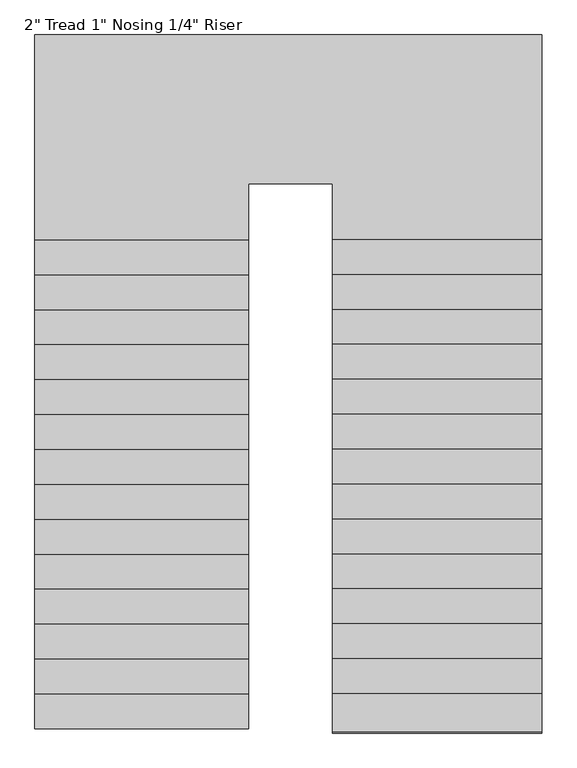
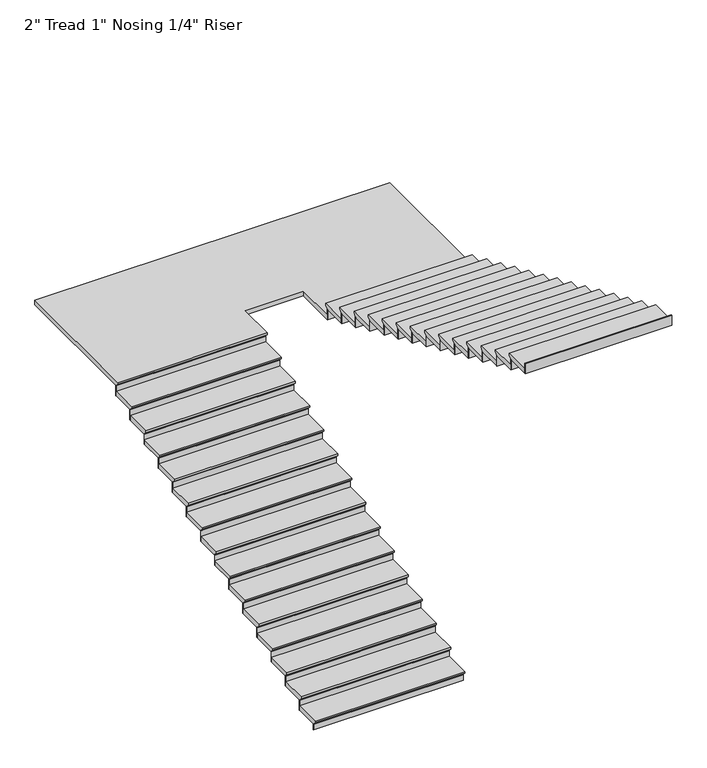
"""IFC4 building model written with IfcOpenShell, lengths in millimetres: stair flight geometry."""

from ifc_helpers import new_model, si_unit, origin, place, context, project, spatial, faceted_brep, source, transform, mapped, element, save


def stair_flight_f7f46773(model_context):
    return source(origin(), model_context, "Body", "Brep", [
        faceted_brep([(-5999.9290366, -6973.0610642, 2835.91), (-5999.9290366, -6973.0610642, 2854.96), (-7554.4415084, -6973.0610642, 2854.96), (-7554.4415084, -6973.0610642, 2835.91), (-5999.9290366, -6947.6610642, 2810.51), (-7554.4415084, -6947.6610642, 2810.51), (-5999.9290366, -6693.6610642, 2854.96), (-7554.4415084, -6693.6610642, 2854.96), (-7554.4415084, -6947.6610642, 2804.16), (-7554.4415084, -6693.6610642, 2804.16), (-5999.9290366, -6693.6610642, 2804.16), (-5999.9290366, -6947.6610642, 2804.16)], [[[0, 1, 2, 3]], [[4, 0, 3, 5]], [[2, 1, 6, 7]], [[8, 9, 10, 11]], [[2, 7, 9, 8, 5, 3]], [[8, 11, 4, 5]], [[6, 1, 0, 4, 11, 10]], [[7, 6, 10, 9]]]),
        faceted_brep([(-5999.9290366, -6947.6610642, 2804.16), (-5999.9290366, -6947.6610642, 2743.2), (-5999.9290366, -6941.3110642, 2743.2), (-5999.9290366, -6941.3110642, 2804.16), (-7554.4415084, -6947.6610642, 2804.16), (-7554.4415084, -6941.3110642, 2804.16), (-7554.4415084, -6941.3110642, 2743.2), (-7554.4415084, -6947.6610642, 2743.2)], [[[0, 1, 2, 3]], [[4, 5, 6, 7]], [[1, 0, 4, 7]], [[2, 1, 7, 6]], [[3, 2, 6, 5]], [[0, 3, 5, 4]]]),
        faceted_brep([(-5999.9290366, -6693.6610642, 2915.92), (-5999.9290366, -6693.6610642, 2804.16), (-5999.9290366, -6687.3110642, 2804.16), (-5999.9290366, -6687.3110642, 2915.92), (-7554.4415084, -6693.6610642, 2915.92), (-7554.4415084, -6687.3110642, 2915.92), (-7554.4415084, -6687.3110642, 2804.16), (-7554.4415084, -6693.6610642, 2804.16)], [[[0, 1, 2, 3]], [[4, 5, 6, 7]], [[1, 0, 4, 7]], [[2, 1, 7, 6]], [[3, 2, 6, 5]], [[0, 3, 5, 4]]]),
        faceted_brep([(-7554.4415084, -6719.0610642, 2966.72), (-5999.9290366, -6719.0610642, 2966.72), (-5999.9290366, -6439.6610642, 2966.72), (-7554.4415084, -6439.6610642, 2966.72), (-7554.4415084, -6693.6610642, 2915.92), (-7554.4415084, -6439.6610642, 2915.92), (-5999.9290366, -6439.6610642, 2915.92), (-5999.9290366, -6693.6610642, 2915.92), (-7554.4415084, -6693.6610642, 2922.27), (-7554.4415084, -6719.0610642, 2947.67), (-5999.9290366, -6693.6610642, 2922.27), (-5999.9290366, -6719.0610642, 2947.67)], [[[0, 1, 2, 3]], [[4, 5, 6, 7]], [[0, 3, 5, 4, 8, 9]], [[4, 7, 10, 8]], [[2, 1, 11, 10, 7, 6]], [[3, 2, 6, 5]], [[11, 1, 0, 9]], [[10, 11, 9, 8]]]),
        faceted_brep([(-5999.9290366, -6439.6610642, 3027.68), (-5999.9290366, -6439.6610642, 2915.92), (-5999.9290366, -6433.3110642, 2915.92), (-5999.9290366, -6433.3110642, 3027.68), (-7554.4415084, -6439.6610642, 3027.68), (-7554.4415084, -6433.3110642, 3027.68), (-7554.4415084, -6433.3110642, 2915.92), (-7554.4415084, -6439.6610642, 2915.92)], [[[0, 1, 2, 3]], [[4, 5, 6, 7]], [[1, 0, 4, 7]], [[2, 1, 7, 6]], [[3, 2, 6, 5]], [[0, 3, 5, 4]]]),
        faceted_brep([(-7554.4415084, -6465.0610642, 3078.48), (-5999.9290366, -6465.0610642, 3078.48), (-5999.9290366, -6185.6610642, 3078.48), (-7554.4415084, -6185.6610642, 3078.48), (-7554.4415084, -6439.6610642, 3027.68), (-7554.4415084, -6185.6610642, 3027.68), (-5999.9290366, -6185.6610642, 3027.68), (-5999.9290366, -6439.6610642, 3027.68), (-7554.4415084, -6439.6610642, 3034.03), (-7554.4415084, -6465.0610642, 3059.43), (-5999.9290366, -6439.6610642, 3034.03), (-5999.9290366, -6465.0610642, 3059.43)], [[[0, 1, 2, 3]], [[4, 5, 6, 7]], [[0, 3, 5, 4, 8, 9]], [[4, 7, 10, 8]], [[2, 1, 11, 10, 7, 6]], [[3, 2, 6, 5]], [[11, 1, 0, 9]], [[10, 11, 9, 8]]]),
        faceted_brep([(-5999.9290366, -6185.6610642, 3139.44), (-5999.9290366, -6185.6610642, 3027.68), (-5999.9290366, -6179.3110642, 3027.68), (-5999.9290366, -6179.3110642, 3139.44), (-7554.4415084, -6185.6610642, 3139.44), (-7554.4415084, -6179.3110642, 3139.44), (-7554.4415084, -6179.3110642, 3027.68), (-7554.4415084, -6185.6610642, 3027.68)], [[[0, 1, 2, 3]], [[4, 5, 6, 7]], [[1, 0, 4, 7]], [[2, 1, 7, 6]], [[3, 2, 6, 5]], [[0, 3, 5, 4]]]),
        faceted_brep([(-7554.4415084, -6211.0610642, 3190.24), (-5999.9290366, -6211.0610642, 3190.24), (-5999.9290366, -5931.6610642, 3190.24), (-7554.4415084, -5931.6610642, 3190.24), (-7554.4415084, -6185.6610642, 3139.44), (-7554.4415084, -5931.6610642, 3139.44), (-5999.9290366, -5931.6610642, 3139.44), (-5999.9290366, -6185.6610642, 3139.44), (-7554.4415084, -6185.6610642, 3145.79), (-7554.4415084, -6211.0610642, 3171.19), (-5999.9290366, -6185.6610642, 3145.79), (-5999.9290366, -6211.0610642, 3171.19)], [[[0, 1, 2, 3]], [[4, 5, 6, 7]], [[0, 3, 5, 4, 8, 9]], [[4, 7, 10, 8]], [[2, 1, 11, 10, 7, 6]], [[3, 2, 6, 5]], [[11, 1, 0, 9]], [[10, 11, 9, 8]]]),
        faceted_brep([(-5999.9290366, -5931.6610642, 3251.2), (-5999.9290366, -5931.6610642, 3139.44), (-5999.9290366, -5925.3110642, 3139.44), (-5999.9290366, -5925.3110642, 3251.2), (-7554.4415084, -5931.6610642, 3251.2), (-7554.4415084, -5925.3110642, 3251.2), (-7554.4415084, -5925.3110642, 3139.44), (-7554.4415084, -5931.6610642, 3139.44)], [[[0, 1, 2, 3]], [[4, 5, 6, 7]], [[1, 0, 4, 7]], [[2, 1, 7, 6]], [[3, 2, 6, 5]], [[0, 3, 5, 4]]]),
        faceted_brep([(-7554.4415084, -5957.0610642, 3302.0), (-5999.9290366, -5957.0610642, 3302.0), (-5999.9290366, -5677.6610642, 3302.0), (-7554.4415084, -5677.6610642, 3302.0), (-7554.4415084, -5931.6610642, 3251.2), (-7554.4415084, -5677.6610642, 3251.2), (-5999.9290366, -5677.6610642, 3251.2), (-5999.9290366, -5931.6610642, 3251.2), (-7554.4415084, -5931.6610642, 3257.55), (-7554.4415084, -5957.0610642, 3282.95), (-5999.9290366, -5931.6610642, 3257.55), (-5999.9290366, -5957.0610642, 3282.95)], [[[0, 1, 2, 3]], [[4, 5, 6, 7]], [[0, 3, 5, 4, 8, 9]], [[4, 7, 10, 8]], [[2, 1, 11, 10, 7, 6]], [[3, 2, 6, 5]], [[11, 1, 0, 9]], [[10, 11, 9, 8]]]),
        faceted_brep([(-5999.9290366, -5677.6610642, 3362.96), (-5999.9290366, -5677.6610642, 3251.2), (-5999.9290366, -5671.3110642, 3251.2), (-5999.9290366, -5671.3110642, 3362.96), (-7554.4415084, -5677.6610642, 3362.96), (-7554.4415084, -5671.3110642, 3362.96), (-7554.4415084, -5671.3110642, 3251.2), (-7554.4415084, -5677.6610642, 3251.2)], [[[0, 1, 2, 3]], [[4, 5, 6, 7]], [[1, 0, 4, 7]], [[2, 1, 7, 6]], [[3, 2, 6, 5]], [[0, 3, 5, 4]]]),
        faceted_brep([(-7554.4415084, -5703.0610642, 3413.76), (-5999.9290366, -5703.0610642, 3413.76), (-5999.9290366, -5423.6610642, 3413.76), (-7554.4415084, -5423.6610642, 3413.76), (-7554.4415084, -5677.6610642, 3362.96), (-7554.4415084, -5423.6610642, 3362.96), (-5999.9290366, -5423.6610642, 3362.96), (-5999.9290366, -5677.6610642, 3362.96), (-7554.4415084, -5677.6610642, 3369.31), (-7554.4415084, -5703.0610642, 3394.71), (-5999.9290366, -5677.6610642, 3369.31), (-5999.9290366, -5703.0610642, 3394.71)], [[[0, 1, 2, 3]], [[4, 5, 6, 7]], [[0, 3, 5, 4, 8, 9]], [[4, 7, 10, 8]], [[2, 1, 11, 10, 7, 6]], [[3, 2, 6, 5]], [[11, 1, 0, 9]], [[10, 11, 9, 8]]]),
        faceted_brep([(-5999.9290366, -5423.6610642, 3474.72), (-5999.9290366, -5423.6610642, 3362.96), (-5999.9290366, -5417.3110642, 3362.96), (-5999.9290366, -5417.3110642, 3474.72), (-7554.4415084, -5423.6610642, 3474.72), (-7554.4415084, -5417.3110642, 3474.72), (-7554.4415084, -5417.3110642, 3362.96), (-7554.4415084, -5423.6610642, 3362.96)], [[[0, 1, 2, 3]], [[4, 5, 6, 7]], [[1, 0, 4, 7]], [[2, 1, 7, 6]], [[3, 2, 6, 5]], [[0, 3, 5, 4]]]),
        faceted_brep([(-7554.4415084, -5449.0610642, 3525.52), (-5999.9290366, -5449.0610642, 3525.52), (-5999.9290366, -5169.6610642, 3525.52), (-7554.4415084, -5169.6610642, 3525.52), (-7554.4415084, -5423.6610642, 3474.72), (-7554.4415084, -5169.6610642, 3474.72), (-5999.9290366, -5169.6610642, 3474.72), (-5999.9290366, -5423.6610642, 3474.72), (-7554.4415084, -5423.6610642, 3481.07), (-7554.4415084, -5449.0610642, 3506.47), (-5999.9290366, -5423.6610642, 3481.07), (-5999.9290366, -5449.0610642, 3506.47)], [[[0, 1, 2, 3]], [[4, 5, 6, 7]], [[0, 3, 5, 4, 8, 9]], [[4, 7, 10, 8]], [[2, 1, 11, 10, 7, 6]], [[3, 2, 6, 5]], [[11, 1, 0, 9]], [[10, 11, 9, 8]]]),
        faceted_brep([(-5999.9290366, -5169.6610642, 3586.48), (-5999.9290366, -5169.6610642, 3474.72), (-5999.9290366, -5163.3110642, 3474.72), (-5999.9290366, -5163.3110642, 3586.48), (-7554.4415084, -5169.6610642, 3586.48), (-7554.4415084, -5163.3110642, 3586.48), (-7554.4415084, -5163.3110642, 3474.72), (-7554.4415084, -5169.6610642, 3474.72)], [[[0, 1, 2, 3]], [[4, 5, 6, 7]], [[1, 0, 4, 7]], [[2, 1, 7, 6]], [[3, 2, 6, 5]], [[0, 3, 5, 4]]]),
        faceted_brep([(-7554.4415084, -5195.0610642, 3637.28), (-5999.9290366, -5195.0610642, 3637.28), (-5999.9290366, -4915.6610642, 3637.28), (-7554.4415084, -4915.6610642, 3637.28), (-7554.4415084, -5169.6610642, 3586.48), (-7554.4415084, -4915.6610642, 3586.48), (-5999.9290366, -4915.6610642, 3586.48), (-5999.9290366, -5169.6610642, 3586.48), (-7554.4415084, -5169.6610642, 3592.83), (-7554.4415084, -5195.0610642, 3618.23), (-5999.9290366, -5169.6610642, 3592.83), (-5999.9290366, -5195.0610642, 3618.23)], [[[0, 1, 2, 3]], [[4, 5, 6, 7]], [[0, 3, 5, 4, 8, 9]], [[4, 7, 10, 8]], [[2, 1, 11, 10, 7, 6]], [[3, 2, 6, 5]], [[11, 1, 0, 9]], [[10, 11, 9, 8]]]),
        faceted_brep([(-5999.9290366, -4915.6610642, 3698.24), (-5999.9290366, -4915.6610642, 3586.48), (-5999.9290366, -4909.3110642, 3586.48), (-5999.9290366, -4909.3110642, 3698.24), (-7554.4415084, -4915.6610642, 3698.24), (-7554.4415084, -4909.3110642, 3698.24), (-7554.4415084, -4909.3110642, 3586.48), (-7554.4415084, -4915.6610642, 3586.48)], [[[0, 1, 2, 3]], [[4, 5, 6, 7]], [[1, 0, 4, 7]], [[2, 1, 7, 6]], [[3, 2, 6, 5]], [[0, 3, 5, 4]]]),
        faceted_brep([(-7554.4415084, -4941.0610642, 3749.04), (-5999.9290366, -4941.0610642, 3749.04), (-5999.9290366, -4661.6610642, 3749.04), (-7554.4415084, -4661.6610642, 3749.04), (-7554.4415084, -4915.6610642, 3698.24), (-7554.4415084, -4661.6610642, 3698.24), (-5999.9290366, -4661.6610642, 3698.24), (-5999.9290366, -4915.6610642, 3698.24), (-7554.4415084, -4915.6610642, 3704.59), (-7554.4415084, -4941.0610642, 3729.99), (-5999.9290366, -4915.6610642, 3704.59), (-5999.9290366, -4941.0610642, 3729.99)], [[[0, 1, 2, 3]], [[4, 5, 6, 7]], [[0, 3, 5, 4, 8, 9]], [[4, 7, 10, 8]], [[2, 1, 11, 10, 7, 6]], [[3, 2, 6, 5]], [[11, 1, 0, 9]], [[10, 11, 9, 8]]]),
        faceted_brep([(-5999.9290366, -4661.6610642, 3810.0), (-5999.9290366, -4661.6610642, 3698.24), (-5999.9290366, -4655.3110642, 3698.24), (-5999.9290366, -4655.3110642, 3810.0), (-7554.4415084, -4661.6610642, 3810.0), (-7554.4415084, -4655.3110642, 3810.0), (-7554.4415084, -4655.3110642, 3698.24), (-7554.4415084, -4661.6610642, 3698.24)], [[[0, 1, 2, 3]], [[4, 5, 6, 7]], [[1, 0, 4, 7]], [[2, 1, 7, 6]], [[3, 2, 6, 5]], [[0, 3, 5, 4]]]),
        faceted_brep([(-7554.4415084, -4687.0610642, 3860.8), (-5999.9290366, -4687.0610642, 3860.8), (-5999.9290366, -4407.6610642, 3860.8), (-7554.4415084, -4407.6610642, 3860.8), (-7554.4415084, -4661.6610642, 3810.0), (-7554.4415084, -4407.6610642, 3810.0), (-5999.9290366, -4407.6610642, 3810.0), (-5999.9290366, -4661.6610642, 3810.0), (-7554.4415084, -4661.6610642, 3816.35), (-7554.4415084, -4687.0610642, 3841.75), (-5999.9290366, -4661.6610642, 3816.35), (-5999.9290366, -4687.0610642, 3841.75)], [[[0, 1, 2, 3]], [[4, 5, 6, 7]], [[0, 3, 5, 4, 8, 9]], [[4, 7, 10, 8]], [[2, 1, 11, 10, 7, 6]], [[3, 2, 6, 5]], [[11, 1, 0, 9]], [[10, 11, 9, 8]]]),
        faceted_brep([(-5999.9290366, -4407.6610642, 3921.76), (-5999.9290366, -4407.6610642, 3810.0), (-5999.9290366, -4401.3110642, 3810.0), (-5999.9290366, -4401.3110642, 3921.76), (-7554.4415084, -4407.6610642, 3921.76), (-7554.4415084, -4401.3110642, 3921.76), (-7554.4415084, -4401.3110642, 3810.0), (-7554.4415084, -4407.6610642, 3810.0)], [[[0, 1, 2, 3]], [[4, 5, 6, 7]], [[1, 0, 4, 7]], [[2, 1, 7, 6]], [[3, 2, 6, 5]], [[0, 3, 5, 4]]]),
        faceted_brep([(-7554.4415084, -4433.0610642, 3972.56), (-5999.9290366, -4433.0610642, 3972.56), (-5999.9290366, -4153.6610642, 3972.56), (-7554.4415084, -4153.6610642, 3972.56), (-7554.4415084, -4407.6610642, 3921.76), (-7554.4415084, -4153.6610642, 3921.76), (-5999.9290366, -4153.6610642, 3921.76), (-5999.9290366, -4407.6610642, 3921.76), (-7554.4415084, -4407.6610642, 3928.11), (-7554.4415084, -4433.0610642, 3953.51), (-5999.9290366, -4407.6610642, 3928.11), (-5999.9290366, -4433.0610642, 3953.51)], [[[0, 1, 2, 3]], [[4, 5, 6, 7]], [[0, 3, 5, 4, 8, 9]], [[4, 7, 10, 8]], [[2, 1, 11, 10, 7, 6]], [[3, 2, 6, 5]], [[11, 1, 0, 9]], [[10, 11, 9, 8]]]),
        faceted_brep([(-5999.9290366, -4153.6610642, 4033.52), (-5999.9290366, -4153.6610642, 3921.76), (-5999.9290366, -4147.3110642, 3921.76), (-5999.9290366, -4147.3110642, 4033.52), (-7554.4415084, -4153.6610642, 4033.52), (-7554.4415084, -4147.3110642, 4033.52), (-7554.4415084, -4147.3110642, 3921.76), (-7554.4415084, -4153.6610642, 3921.76)], [[[0, 1, 2, 3]], [[4, 5, 6, 7]], [[1, 0, 4, 7]], [[2, 1, 7, 6]], [[3, 2, 6, 5]], [[0, 3, 5, 4]]]),
        faceted_brep([(-7554.4415084, -4179.0610642, 4084.32), (-5999.9290366, -4179.0610642, 4084.32), (-5999.9290366, -3899.6610642, 4084.32), (-7554.4415084, -3899.6610642, 4084.32), (-7554.4415084, -4153.6610642, 4033.52), (-7554.4415084, -3899.6610642, 4033.52), (-5999.9290366, -3899.6610642, 4033.52), (-5999.9290366, -4153.6610642, 4033.52), (-7554.4415084, -4153.6610642, 4039.87), (-7554.4415084, -4179.0610642, 4065.27), (-5999.9290366, -4153.6610642, 4039.87), (-5999.9290366, -4179.0610642, 4065.27)], [[[0, 1, 2, 3]], [[4, 5, 6, 7]], [[0, 3, 5, 4, 8, 9]], [[4, 7, 10, 8]], [[2, 1, 11, 10, 7, 6]], [[3, 2, 6, 5]], [[11, 1, 0, 9]], [[10, 11, 9, 8]]]),
        faceted_brep([(-5999.9290366, -3899.6610642, 4145.28), (-5999.9290366, -3899.6610642, 4033.52), (-5999.9290366, -3893.3110642, 4033.52), (-5999.9290366, -3893.3110642, 4145.28), (-7554.4415084, -3899.6610642, 4145.28), (-7554.4415084, -3893.3110642, 4145.28), (-7554.4415084, -3893.3110642, 4033.52), (-7554.4415084, -3899.6610642, 4033.52)], [[[0, 1, 2, 3]], [[4, 5, 6, 7]], [[1, 0, 4, 7]], [[2, 1, 7, 6]], [[3, 2, 6, 5]], [[0, 3, 5, 4]]]),
        faceted_brep([(-7554.4415084, -3925.0610642, 4196.08), (-5999.9290366, -3925.0610642, 4196.08), (-5999.9290366, -3645.6610642, 4196.08), (-7554.4415084, -3645.6610642, 4196.08), (-7554.4415084, -3899.6610642, 4145.28), (-7554.4415084, -3645.6610642, 4145.28), (-5999.9290366, -3645.6610642, 4145.28), (-5999.9290366, -3899.6610642, 4145.28), (-7554.4415084, -3899.6610642, 4151.63), (-7554.4415084, -3925.0610642, 4177.03), (-5999.9290366, -3899.6610642, 4151.63), (-5999.9290366, -3925.0610642, 4177.03)], [[[0, 1, 2, 3]], [[4, 5, 6, 7]], [[0, 3, 5, 4, 8, 9]], [[4, 7, 10, 8]], [[2, 1, 11, 10, 7, 6]], [[3, 2, 6, 5]], [[11, 1, 0, 9]], [[10, 11, 9, 8]]]),
        faceted_brep([(-5999.9290366, -3645.6610642, 4257.04), (-5999.9290366, -3645.6610642, 4145.28), (-5999.9290366, -3639.3110642, 4145.28), (-5999.9290366, -3639.3110642, 4257.04), (-7554.4415084, -3645.6610642, 4257.04), (-7554.4415084, -3639.3110642, 4257.04), (-7554.4415084, -3639.3110642, 4145.28), (-7554.4415084, -3645.6610642, 4145.28)], [[[0, 1, 2, 3]], [[4, 5, 6, 7]], [[1, 0, 4, 7]], [[2, 1, 7, 6]], [[3, 2, 6, 5]], [[0, 3, 5, 4]]]),
        faceted_brep([(-7554.4415084, -3671.0610642, 4307.84), (-5999.9290366, -3671.0610642, 4307.84), (-5999.9290366, -3391.6610642, 4307.84), (-7554.4415084, -3391.6610642, 4307.84), (-7554.4415084, -3645.6610642, 4257.04), (-7554.4415084, -3391.6610642, 4257.04), (-5999.9290366, -3391.6610642, 4257.04), (-5999.9290366, -3645.6610642, 4257.04), (-7554.4415084, -3645.6610642, 4263.39), (-7554.4415084, -3671.0610642, 4288.79), (-5999.9290366, -3645.6610642, 4263.39), (-5999.9290366, -3671.0610642, 4288.79)], [[[0, 1, 2, 3]], [[4, 5, 6, 7]], [[0, 3, 5, 4, 8, 9]], [[4, 7, 10, 8]], [[2, 1, 11, 10, 7, 6]], [[3, 2, 6, 5]], [[11, 1, 0, 9]], [[10, 11, 9, 8]]]),
        faceted_brep([(-5999.9290366, -3391.6610642, 4368.8), (-5999.9290366, -3391.6610642, 4257.04), (-5999.9290366, -3385.3110642, 4257.04), (-5999.9290366, -3385.3110642, 4368.8), (-7554.4415084, -3391.6610642, 4368.8), (-7554.4415084, -3385.3110642, 4368.8), (-7554.4415084, -3385.3110642, 4257.04), (-7554.4415084, -3391.6610642, 4257.04)], [[[0, 1, 2, 3]], [[4, 5, 6, 7]], [[1, 0, 4, 7]], [[2, 1, 7, 6]], [[3, 2, 6, 5]], [[0, 3, 5, 4]]]),
        faceted_brep([(-3866.3290366, -3442.4610642, 4419.6), (-3866.3290366, -1928.4217109, 4419.6), (-7554.4415084, -1928.4217109, 4419.6), (-7554.4415084, -3417.0610642, 4419.6), (-5999.9290366, -3417.0610642, 4419.6), (-5999.9290366, -3010.6610642, 4419.6), (-5390.3290366, -3010.6610642, 4419.6), (-5390.3290366, -3442.4610642, 4419.6), (-3866.3290366, -1928.4217109, 4368.8), (-3866.3290366, -3442.4610642, 4368.8), (-5390.3290366, -3442.4610642, 4368.8), (-5390.3290366, -3010.6610642, 4368.8), (-5999.9290366, -3010.6610642, 4368.8), (-5999.9290366, -3391.6610642, 4368.8), (-7554.4415084, -3391.6610642, 4368.8), (-7554.4415084, -1928.4217109, 4368.8), (-7554.4415084, -3391.6610642, 4375.15), (-7554.4415084, -3417.0610642, 4400.55), (-5999.9290366, -3391.6610642, 4375.15), (-5999.9290366, -3417.0610642, 4400.55)], [[[0, 1, 2, 3, 4, 5, 6, 7]], [[8, 9, 10, 11, 12, 13, 14, 15]], [[1, 0, 9, 8]], [[2, 1, 8, 15]], [[3, 2, 15, 14, 16, 17]], [[14, 13, 18, 16]], [[5, 4, 19, 18, 13, 12]], [[6, 5, 12, 11]], [[7, 6, 11, 10]], [[0, 7, 10, 9]], [[19, 4, 3, 17]], [[18, 19, 17, 16]]]),
        faceted_brep([(-5390.3290366, -3442.4610642, 4480.56), (-5390.3290366, -3442.4610642, 4368.8), (-5390.3290366, -3448.8110642, 4368.8), (-5390.3290366, -3448.8110642, 4480.56), (-3866.3290366, -3442.4610642, 4480.56), (-3866.3290366, -3448.8110642, 4480.56), (-3866.3290366, -3448.8110642, 4368.8), (-3866.3290366, -3442.4610642, 4368.8)], [[[0, 1, 2, 3]], [[4, 5, 6, 7]], [[1, 0, 4, 7]], [[2, 1, 7, 6]], [[3, 2, 6, 5]], [[0, 3, 5, 4]]]),
        faceted_brep([(-3866.3290366, -3417.0610642, 4531.36), (-5390.3290366, -3417.0610642, 4531.36), (-5390.3290366, -3696.4610642, 4531.36), (-3866.3290366, -3696.4610642, 4531.36), (-3866.3290366, -3442.4610642, 4480.56), (-3866.3290366, -3696.4610642, 4480.56), (-5390.3290366, -3696.4610642, 4480.56), (-5390.3290366, -3442.4610642, 4480.56), (-3866.3290366, -3442.4610642, 4486.91), (-3866.3290366, -3417.0610642, 4512.31), (-5390.3290366, -3442.4610642, 4486.91), (-5390.3290366, -3417.0610642, 4512.31)], [[[0, 1, 2, 3]], [[4, 5, 6, 7]], [[0, 3, 5, 4, 8, 9]], [[4, 7, 10, 8]], [[2, 1, 11, 10, 7, 6]], [[3, 2, 6, 5]], [[11, 1, 0, 9]], [[10, 11, 9, 8]]]),
        faceted_brep([(-5390.3290366, -3696.4610642, 4592.32), (-5390.3290366, -3696.4610642, 4480.56), (-5390.3290366, -3702.8110642, 4480.56), (-5390.3290366, -3702.8110642, 4592.32), (-3866.3290366, -3696.4610642, 4592.32), (-3866.3290366, -3702.8110642, 4592.32), (-3866.3290366, -3702.8110642, 4480.56), (-3866.3290366, -3696.4610642, 4480.56)], [[[0, 1, 2, 3]], [[4, 5, 6, 7]], [[1, 0, 4, 7]], [[2, 1, 7, 6]], [[3, 2, 6, 5]], [[0, 3, 5, 4]]]),
        faceted_brep([(-3866.3290366, -3671.0610642, 4643.12), (-5390.3290366, -3671.0610642, 4643.12), (-5390.3290366, -3950.4610642, 4643.12), (-3866.3290366, -3950.4610642, 4643.12), (-3866.3290366, -3696.4610642, 4592.32), (-3866.3290366, -3950.4610642, 4592.32), (-5390.3290366, -3950.4610642, 4592.32), (-5390.3290366, -3696.4610642, 4592.32), (-3866.3290366, -3696.4610642, 4598.67), (-3866.3290366, -3671.0610642, 4624.07), (-5390.3290366, -3696.4610642, 4598.67), (-5390.3290366, -3671.0610642, 4624.07)], [[[0, 1, 2, 3]], [[4, 5, 6, 7]], [[0, 3, 5, 4, 8, 9]], [[4, 7, 10, 8]], [[2, 1, 11, 10, 7, 6]], [[3, 2, 6, 5]], [[11, 1, 0, 9]], [[10, 11, 9, 8]]]),
        faceted_brep([(-5390.3290366, -3950.4610642, 4704.08), (-5390.3290366, -3950.4610642, 4592.32), (-5390.3290366, -3956.8110642, 4592.32), (-5390.3290366, -3956.8110642, 4704.08), (-3866.3290366, -3950.4610642, 4704.08), (-3866.3290366, -3956.8110642, 4704.08), (-3866.3290366, -3956.8110642, 4592.32), (-3866.3290366, -3950.4610642, 4592.32)], [[[0, 1, 2, 3]], [[4, 5, 6, 7]], [[1, 0, 4, 7]], [[2, 1, 7, 6]], [[3, 2, 6, 5]], [[0, 3, 5, 4]]]),
        faceted_brep([(-3866.3290366, -3925.0610642, 4754.88), (-5390.3290366, -3925.0610642, 4754.88), (-5390.3290366, -4204.4610642, 4754.88), (-3866.3290366, -4204.4610642, 4754.88), (-3866.3290366, -3950.4610642, 4704.08), (-3866.3290366, -4204.4610642, 4704.08), (-5390.3290366, -4204.4610642, 4704.08), (-5390.3290366, -3950.4610642, 4704.08), (-3866.3290366, -3950.4610642, 4710.43), (-3866.3290366, -3925.0610642, 4735.83), (-5390.3290366, -3950.4610642, 4710.43), (-5390.3290366, -3925.0610642, 4735.83)], [[[0, 1, 2, 3]], [[4, 5, 6, 7]], [[0, 3, 5, 4, 8, 9]], [[4, 7, 10, 8]], [[2, 1, 11, 10, 7, 6]], [[3, 2, 6, 5]], [[11, 1, 0, 9]], [[10, 11, 9, 8]]]),
        faceted_brep([(-5390.3290366, -4204.4610642, 4815.84), (-5390.3290366, -4204.4610642, 4704.08), (-5390.3290366, -4210.8110642, 4704.08), (-5390.3290366, -4210.8110642, 4815.84), (-3866.3290366, -4204.4610642, 4815.84), (-3866.3290366, -4210.8110642, 4815.84), (-3866.3290366, -4210.8110642, 4704.08), (-3866.3290366, -4204.4610642, 4704.08)], [[[0, 1, 2, 3]], [[4, 5, 6, 7]], [[1, 0, 4, 7]], [[2, 1, 7, 6]], [[3, 2, 6, 5]], [[0, 3, 5, 4]]]),
        faceted_brep([(-3866.3290366, -4179.0610642, 4866.64), (-5390.3290366, -4179.0610642, 4866.64), (-5390.3290366, -4458.4610642, 4866.64), (-3866.3290366, -4458.4610642, 4866.64), (-3866.3290366, -4204.4610642, 4815.84), (-3866.3290366, -4458.4610642, 4815.84), (-5390.3290366, -4458.4610642, 4815.84), (-5390.3290366, -4204.4610642, 4815.84), (-3866.3290366, -4204.4610642, 4822.19), (-3866.3290366, -4179.0610642, 4847.59), (-5390.3290366, -4204.4610642, 4822.19), (-5390.3290366, -4179.0610642, 4847.59)], [[[0, 1, 2, 3]], [[4, 5, 6, 7]], [[0, 3, 5, 4, 8, 9]], [[4, 7, 10, 8]], [[2, 1, 11, 10, 7, 6]], [[3, 2, 6, 5]], [[11, 1, 0, 9]], [[10, 11, 9, 8]]]),
        faceted_brep([(-5390.3290366, -4458.4610642, 4927.6), (-5390.3290366, -4458.4610642, 4815.84), (-5390.3290366, -4464.8110642, 4815.84), (-5390.3290366, -4464.8110642, 4927.6), (-3866.3290366, -4458.4610642, 4927.6), (-3866.3290366, -4464.8110642, 4927.6), (-3866.3290366, -4464.8110642, 4815.84), (-3866.3290366, -4458.4610642, 4815.84)], [[[0, 1, 2, 3]], [[4, 5, 6, 7]], [[1, 0, 4, 7]], [[2, 1, 7, 6]], [[3, 2, 6, 5]], [[0, 3, 5, 4]]]),
        faceted_brep([(-3866.3290366, -4433.0610642, 4978.4), (-5390.3290366, -4433.0610642, 4978.4), (-5390.3290366, -4712.4610642, 4978.4), (-3866.3290366, -4712.4610642, 4978.4), (-3866.3290366, -4458.4610642, 4927.6), (-3866.3290366, -4712.4610642, 4927.6), (-5390.3290366, -4712.4610642, 4927.6), (-5390.3290366, -4458.4610642, 4927.6), (-3866.3290366, -4458.4610642, 4933.95), (-3866.3290366, -4433.0610642, 4959.35), (-5390.3290366, -4458.4610642, 4933.95), (-5390.3290366, -4433.0610642, 4959.35)], [[[0, 1, 2, 3]], [[4, 5, 6, 7]], [[0, 3, 5, 4, 8, 9]], [[4, 7, 10, 8]], [[2, 1, 11, 10, 7, 6]], [[3, 2, 6, 5]], [[11, 1, 0, 9]], [[10, 11, 9, 8]]]),
        faceted_brep([(-5390.3290366, -4712.4610642, 5039.36), (-5390.3290366, -4712.4610642, 4927.6), (-5390.3290366, -4718.8110642, 4927.6), (-5390.3290366, -4718.8110642, 5039.36), (-3866.3290366, -4712.4610642, 5039.36), (-3866.3290366, -4718.8110642, 5039.36), (-3866.3290366, -4718.8110642, 4927.6), (-3866.3290366, -4712.4610642, 4927.6)], [[[0, 1, 2, 3]], [[4, 5, 6, 7]], [[1, 0, 4, 7]], [[2, 1, 7, 6]], [[3, 2, 6, 5]], [[0, 3, 5, 4]]]),
        faceted_brep([(-3866.3290366, -4687.0610642, 5090.16), (-5390.3290366, -4687.0610642, 5090.16), (-5390.3290366, -4966.4610642, 5090.16), (-3866.3290366, -4966.4610642, 5090.16), (-3866.3290366, -4712.4610642, 5039.36), (-3866.3290366, -4966.4610642, 5039.36), (-5390.3290366, -4966.4610642, 5039.36), (-5390.3290366, -4712.4610642, 5039.36), (-3866.3290366, -4712.4610642, 5045.71), (-3866.3290366, -4687.0610642, 5071.11), (-5390.3290366, -4712.4610642, 5045.71), (-5390.3290366, -4687.0610642, 5071.11)], [[[0, 1, 2, 3]], [[4, 5, 6, 7]], [[0, 3, 5, 4, 8, 9]], [[4, 7, 10, 8]], [[2, 1, 11, 10, 7, 6]], [[3, 2, 6, 5]], [[11, 1, 0, 9]], [[10, 11, 9, 8]]]),
        faceted_brep([(-5390.3290366, -4966.4610642, 5151.12), (-5390.3290366, -4966.4610642, 5039.36), (-5390.3290366, -4972.8110642, 5039.36), (-5390.3290366, -4972.8110642, 5151.12), (-3866.3290366, -4966.4610642, 5151.12), (-3866.3290366, -4972.8110642, 5151.12), (-3866.3290366, -4972.8110642, 5039.36), (-3866.3290366, -4966.4610642, 5039.36)], [[[0, 1, 2, 3]], [[4, 5, 6, 7]], [[1, 0, 4, 7]], [[2, 1, 7, 6]], [[3, 2, 6, 5]], [[0, 3, 5, 4]]]),
        faceted_brep([(-3866.3290366, -4941.0610642, 5201.92), (-5390.3290366, -4941.0610642, 5201.92), (-5390.3290366, -5220.4610642, 5201.92), (-3866.3290366, -5220.4610642, 5201.92), (-3866.3290366, -4966.4610642, 5151.12), (-3866.3290366, -5220.4610642, 5151.12), (-5390.3290366, -5220.4610642, 5151.12), (-5390.3290366, -4966.4610642, 5151.12), (-3866.3290366, -4966.4610642, 5157.47), (-3866.3290366, -4941.0610642, 5182.87), (-5390.3290366, -4966.4610642, 5157.47), (-5390.3290366, -4941.0610642, 5182.87)], [[[0, 1, 2, 3]], [[4, 5, 6, 7]], [[0, 3, 5, 4, 8, 9]], [[4, 7, 10, 8]], [[2, 1, 11, 10, 7, 6]], [[3, 2, 6, 5]], [[11, 1, 0, 9]], [[10, 11, 9, 8]]]),
        faceted_brep([(-5390.3290366, -5220.4610642, 5262.88), (-5390.3290366, -5220.4610642, 5151.12), (-5390.3290366, -5226.8110642, 5151.12), (-5390.3290366, -5226.8110642, 5262.88), (-3866.3290366, -5220.4610642, 5262.88), (-3866.3290366, -5226.8110642, 5262.88), (-3866.3290366, -5226.8110642, 5151.12), (-3866.3290366, -5220.4610642, 5151.12)], [[[0, 1, 2, 3]], [[4, 5, 6, 7]], [[1, 0, 4, 7]], [[2, 1, 7, 6]], [[3, 2, 6, 5]], [[0, 3, 5, 4]]]),
        faceted_brep([(-3866.3290366, -5195.0610642, 5313.68), (-5390.3290366, -5195.0610642, 5313.68), (-5390.3290366, -5474.4610642, 5313.68), (-3866.3290366, -5474.4610642, 5313.68), (-3866.3290366, -5220.4610642, 5262.88), (-3866.3290366, -5474.4610642, 5262.88), (-5390.3290366, -5474.4610642, 5262.88), (-5390.3290366, -5220.4610642, 5262.88), (-3866.3290366, -5220.4610642, 5269.23), (-3866.3290366, -5195.0610642, 5294.63), (-5390.3290366, -5220.4610642, 5269.23), (-5390.3290366, -5195.0610642, 5294.63)], [[[0, 1, 2, 3]], [[4, 5, 6, 7]], [[0, 3, 5, 4, 8, 9]], [[4, 7, 10, 8]], [[2, 1, 11, 10, 7, 6]], [[3, 2, 6, 5]], [[11, 1, 0, 9]], [[10, 11, 9, 8]]]),
        faceted_brep([(-5390.3290366, -5474.4610642, 5374.64), (-5390.3290366, -5474.4610642, 5262.88), (-5390.3290366, -5480.8110642, 5262.88), (-5390.3290366, -5480.8110642, 5374.64), (-3866.3290366, -5474.4610642, 5374.64), (-3866.3290366, -5480.8110642, 5374.64), (-3866.3290366, -5480.8110642, 5262.88), (-3866.3290366, -5474.4610642, 5262.88)], [[[0, 1, 2, 3]], [[4, 5, 6, 7]], [[1, 0, 4, 7]], [[2, 1, 7, 6]], [[3, 2, 6, 5]], [[0, 3, 5, 4]]]),
        faceted_brep([(-3866.3290366, -5449.0610642, 5425.44), (-5390.3290366, -5449.0610642, 5425.44), (-5390.3290366, -5728.4610642, 5425.44), (-3866.3290366, -5728.4610642, 5425.44), (-3866.3290366, -5474.4610642, 5374.64), (-3866.3290366, -5728.4610642, 5374.64), (-5390.3290366, -5728.4610642, 5374.64), (-5390.3290366, -5474.4610642, 5374.64), (-3866.3290366, -5474.4610642, 5380.99), (-3866.3290366, -5449.0610642, 5406.39), (-5390.3290366, -5474.4610642, 5380.99), (-5390.3290366, -5449.0610642, 5406.39)], [[[0, 1, 2, 3]], [[4, 5, 6, 7]], [[0, 3, 5, 4, 8, 9]], [[4, 7, 10, 8]], [[2, 1, 11, 10, 7, 6]], [[3, 2, 6, 5]], [[11, 1, 0, 9]], [[10, 11, 9, 8]]]),
        faceted_brep([(-5390.3290366, -5728.4610642, 5486.4), (-5390.3290366, -5728.4610642, 5374.64), (-5390.3290366, -5734.8110642, 5374.64), (-5390.3290366, -5734.8110642, 5486.4), (-3866.3290366, -5728.4610642, 5486.4), (-3866.3290366, -5734.8110642, 5486.4), (-3866.3290366, -5734.8110642, 5374.64), (-3866.3290366, -5728.4610642, 5374.64)], [[[0, 1, 2, 3]], [[4, 5, 6, 7]], [[1, 0, 4, 7]], [[2, 1, 7, 6]], [[3, 2, 6, 5]], [[0, 3, 5, 4]]]),
        faceted_brep([(-3866.3290366, -5703.0610642, 5537.2), (-5390.3290366, -5703.0610642, 5537.2), (-5390.3290366, -5982.4610642, 5537.2), (-3866.3290366, -5982.4610642, 5537.2), (-3866.3290366, -5728.4610642, 5486.4), (-3866.3290366, -5982.4610642, 5486.4), (-5390.3290366, -5982.4610642, 5486.4), (-5390.3290366, -5728.4610642, 5486.4), (-3866.3290366, -5728.4610642, 5492.75), (-3866.3290366, -5703.0610642, 5518.15), (-5390.3290366, -5728.4610642, 5492.75), (-5390.3290366, -5703.0610642, 5518.15)], [[[0, 1, 2, 3]], [[4, 5, 6, 7]], [[0, 3, 5, 4, 8, 9]], [[4, 7, 10, 8]], [[2, 1, 11, 10, 7, 6]], [[3, 2, 6, 5]], [[11, 1, 0, 9]], [[10, 11, 9, 8]]]),
        faceted_brep([(-5390.3290366, -5982.4610642, 5598.16), (-5390.3290366, -5982.4610642, 5486.4), (-5390.3290366, -5988.8110642, 5486.4), (-5390.3290366, -5988.8110642, 5598.16), (-3866.3290366, -5982.4610642, 5598.16), (-3866.3290366, -5988.8110642, 5598.16), (-3866.3290366, -5988.8110642, 5486.4), (-3866.3290366, -5982.4610642, 5486.4)], [[[0, 1, 2, 3]], [[4, 5, 6, 7]], [[1, 0, 4, 7]], [[2, 1, 7, 6]], [[3, 2, 6, 5]], [[0, 3, 5, 4]]]),
        faceted_brep([(-3866.3290366, -5957.0610642, 5648.96), (-5390.3290366, -5957.0610642, 5648.96), (-5390.3290366, -6236.4610642, 5648.96), (-3866.3290366, -6236.4610642, 5648.96), (-3866.3290366, -5982.4610642, 5598.16), (-3866.3290366, -6236.4610642, 5598.16), (-5390.3290366, -6236.4610642, 5598.16), (-5390.3290366, -5982.4610642, 5598.16), (-3866.3290366, -5982.4610642, 5604.51), (-3866.3290366, -5957.0610642, 5629.91), (-5390.3290366, -5982.4610642, 5604.51), (-5390.3290366, -5957.0610642, 5629.91)], [[[0, 1, 2, 3]], [[4, 5, 6, 7]], [[0, 3, 5, 4, 8, 9]], [[4, 7, 10, 8]], [[2, 1, 11, 10, 7, 6]], [[3, 2, 6, 5]], [[11, 1, 0, 9]], [[10, 11, 9, 8]]]),
        faceted_brep([(-5390.3290366, -6236.4610642, 5709.92), (-5390.3290366, -6236.4610642, 5598.16), (-5390.3290366, -6242.8110642, 5598.16), (-5390.3290366, -6242.8110642, 5709.92), (-3866.3290366, -6236.4610642, 5709.92), (-3866.3290366, -6242.8110642, 5709.92), (-3866.3290366, -6242.8110642, 5598.16), (-3866.3290366, -6236.4610642, 5598.16)], [[[0, 1, 2, 3]], [[4, 5, 6, 7]], [[1, 0, 4, 7]], [[2, 1, 7, 6]], [[3, 2, 6, 5]], [[0, 3, 5, 4]]]),
        faceted_brep([(-3866.3290366, -6211.0610642, 5760.72), (-5390.3290366, -6211.0610642, 5760.72), (-5390.3290366, -6490.4610642, 5760.72), (-3866.3290366, -6490.4610642, 5760.72), (-3866.3290366, -6236.4610642, 5709.92), (-3866.3290366, -6490.4610642, 5709.92), (-5390.3290366, -6490.4610642, 5709.92), (-5390.3290366, -6236.4610642, 5709.92), (-3866.3290366, -6236.4610642, 5716.27), (-3866.3290366, -6211.0610642, 5741.67), (-5390.3290366, -6236.4610642, 5716.27), (-5390.3290366, -6211.0610642, 5741.67)], [[[0, 1, 2, 3]], [[4, 5, 6, 7]], [[0, 3, 5, 4, 8, 9]], [[4, 7, 10, 8]], [[2, 1, 11, 10, 7, 6]], [[3, 2, 6, 5]], [[11, 1, 0, 9]], [[10, 11, 9, 8]]]),
        faceted_brep([(-5390.3290366, -6490.4610642, 5821.68), (-5390.3290366, -6490.4610642, 5709.92), (-5390.3290366, -6496.8110642, 5709.92), (-5390.3290366, -6496.8110642, 5821.68), (-3866.3290366, -6490.4610642, 5821.68), (-3866.3290366, -6496.8110642, 5821.68), (-3866.3290366, -6496.8110642, 5709.92), (-3866.3290366, -6490.4610642, 5709.92)], [[[0, 1, 2, 3]], [[4, 5, 6, 7]], [[1, 0, 4, 7]], [[2, 1, 7, 6]], [[3, 2, 6, 5]], [[0, 3, 5, 4]]]),
        faceted_brep([(-3866.3290366, -6465.0610642, 5872.48), (-5390.3290366, -6465.0610642, 5872.48), (-5390.3290366, -6744.4610642, 5872.48), (-3866.3290366, -6744.4610642, 5872.48), (-3866.3290366, -6490.4610642, 5821.68), (-3866.3290366, -6744.4610642, 5821.68), (-5390.3290366, -6744.4610642, 5821.68), (-5390.3290366, -6490.4610642, 5821.68), (-3866.3290366, -6490.4610642, 5828.03), (-3866.3290366, -6465.0610642, 5853.43), (-5390.3290366, -6490.4610642, 5828.03), (-5390.3290366, -6465.0610642, 5853.43)], [[[0, 1, 2, 3]], [[4, 5, 6, 7]], [[0, 3, 5, 4, 8, 9]], [[4, 7, 10, 8]], [[2, 1, 11, 10, 7, 6]], [[3, 2, 6, 5]], [[11, 1, 0, 9]], [[10, 11, 9, 8]]]),
        faceted_brep([(-5390.3290366, -6744.4610642, 5933.44), (-5390.3290366, -6744.4610642, 5821.68), (-5390.3290366, -6750.8110642, 5821.68), (-5390.3290366, -6750.8110642, 5933.44), (-3866.3290366, -6744.4610642, 5933.44), (-3866.3290366, -6750.8110642, 5933.44), (-3866.3290366, -6750.8110642, 5821.68), (-3866.3290366, -6744.4610642, 5821.68)], [[[0, 1, 2, 3]], [[4, 5, 6, 7]], [[1, 0, 4, 7]], [[2, 1, 7, 6]], [[3, 2, 6, 5]], [[0, 3, 5, 4]]]),
        faceted_brep([(-5390.3290366, -6998.4610642, 6045.2), (-5390.3290366, -6998.4610642, 5933.44), (-5390.3290366, -7004.8110642, 5933.44), (-5390.3290366, -7004.8110642, 6045.2), (-3866.3290366, -6998.4610642, 6045.2), (-3866.3290366, -7004.8110642, 6045.2), (-3866.3290366, -7004.8110642, 5933.44), (-3866.3290366, -6998.4610642, 5933.44)], [[[0, 1, 2, 3]], [[4, 5, 6, 7]], [[1, 0, 4, 7]], [[2, 1, 7, 6]], [[3, 2, 6, 5]], [[0, 3, 5, 4]]]),
        faceted_brep([(-3866.3290366, -6719.0610642, 5984.24), (-5390.3290366, -6719.0610642, 5984.24), (-5390.3290366, -6998.4610642, 5984.24), (-3866.3290366, -6998.4610642, 5984.24), (-3866.3290366, -6744.4610642, 5933.44), (-3866.3290366, -6998.4610642, 5933.44), (-5390.3290366, -6998.4610642, 5933.44), (-5390.3290366, -6744.4610642, 5933.44), (-3866.3290366, -6744.4610642, 5939.79), (-3866.3290366, -6719.0610642, 5965.19), (-5390.3290366, -6744.4610642, 5939.79), (-5390.3290366, -6719.0610642, 5965.19)], [[[0, 1, 2, 3]], [[4, 5, 6, 7]], [[0, 3, 5, 4, 8, 9]], [[4, 7, 10, 8]], [[2, 1, 11, 10, 7, 6]], [[3, 2, 6, 5]], [[11, 1, 0, 9]], [[10, 11, 9, 8]]]),
    ])


if __name__ == "__main__":
    model = new_model("IFC4")
    model_context = context("Model", 3, world=origin())
    ifc_project = project(units=[si_unit("LENGTHUNIT", "METRE", prefix="MILLI")], contexts=[model_context])
    site = spatial("IfcSite", under=ifc_project)
    building = spatial("IfcBuilding", under=site)
    placement = place(None, origin())
    stair_flight_shape = stair_flight_f7f46773(model_context)
    element("IfcStairFlight", 1, ObjectType="2\" Tread 1\" Nosing 1/4\" Riser", at=placement, inside=building, context=model_context, shape_type="MappedRepresentation", body=[
        mapped(stair_flight_shape, transform((0.0, 0.0, 0.0), x_axis=(1.0, 0.0, 0.0), y_axis=(0.0, 1.0, 0.0), z_axis=(0.0, 0.0, 1.0))),
    ])
    save(model, "model.ifc")
